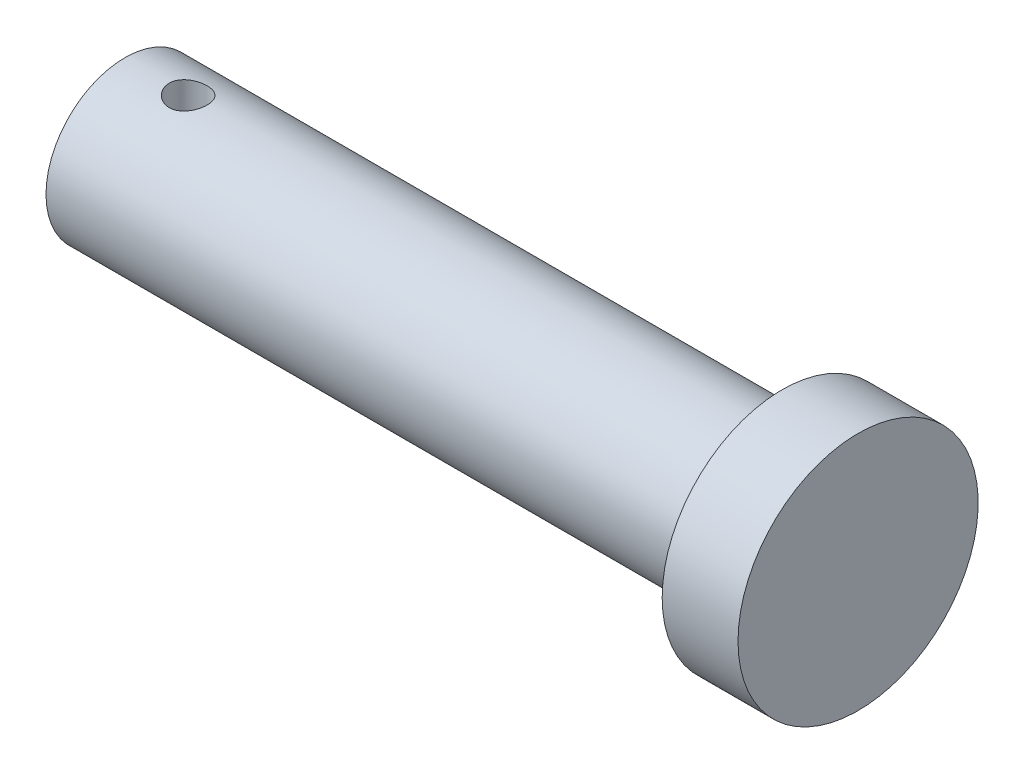
SolidWorks part; units mm, degrees
material "Plain Carbon Steel"
ref_plane "Front Plane" through (0, 0, 0) normal (0, 0, 1) x (1, 0, 0)
ref_plane "Top Plane" through (0, 0, 0) normal (0, 1, 0) x (1, 0, 0)
ref_plane "Right Plane" through (0, 0, 0) normal (1, 0, 0) x (0, 0, -1)
sketch "Pin Profile Sketch" plane through (0, 0, 0) normal (0, 0, 1) x (1, 0, 0)
  line L0 (-210, 0) -> (211.7746, 0) construction
  line L1 (0, 104.2606) -> (0, -108.6972) construction
  line L3 (0, 0) -> (84, 0)
  line L4 (0, 0) -> (0, -12.5)
  line L5 (0, -12.5) -> (104, -12.5)
  line L7 (84, 0) -> (116, 0)
  line L8 (104, -12.5) -> (104, -19)
  line L9 (104, -19) -> (116, -19)
  line L10 (116, 0) -> (116, -19)
  dimension "D1" = 104
  dimension "D2" = 12
  dimension "D3" = 12.5
  dimension "D4" = 19
  dimension "D5" = 84
revolve "Headed Pin Body" add sketch "Pin Profile Sketch" angle 360 about L0
sketch "Cross Hole Sketch" plane through (0, 0, 0) normal (0, 1, 0) x (1, 0, 0)
  circle A0 centre (10, 0) radius 3
  dimension "D1" = 6
  dimension "D2" = 10
extrude "Cross Hole Ø6" cut sketch "Cross Hole Sketch" against normal through all both and the other way through all
